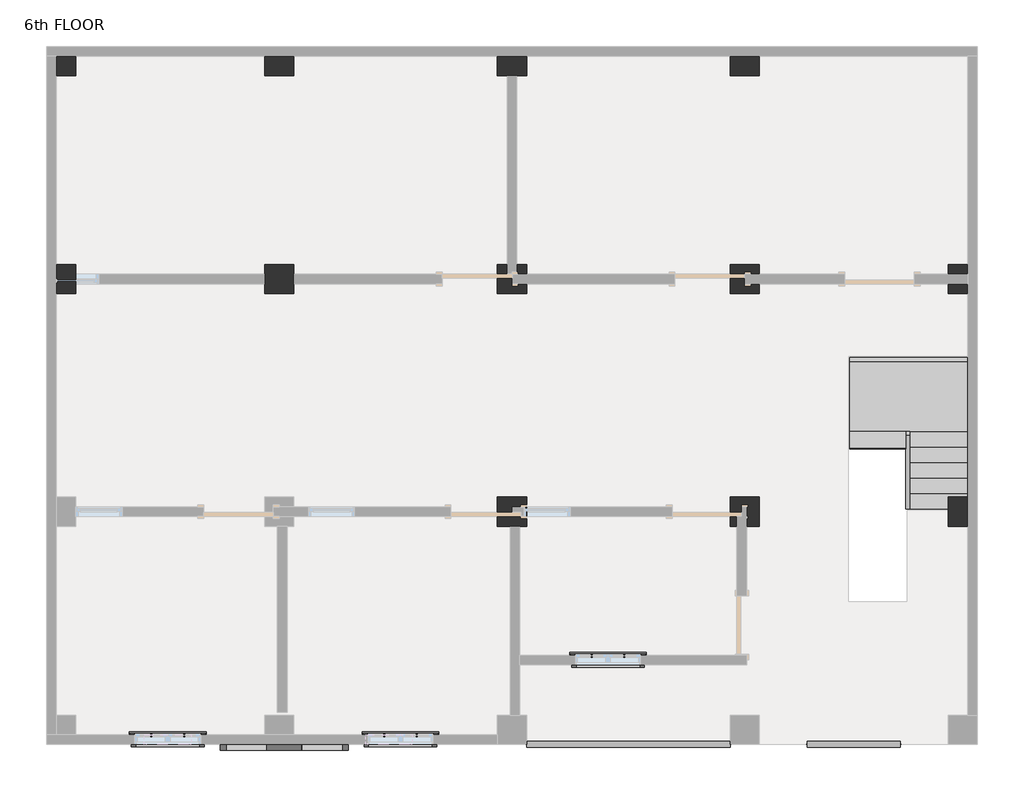
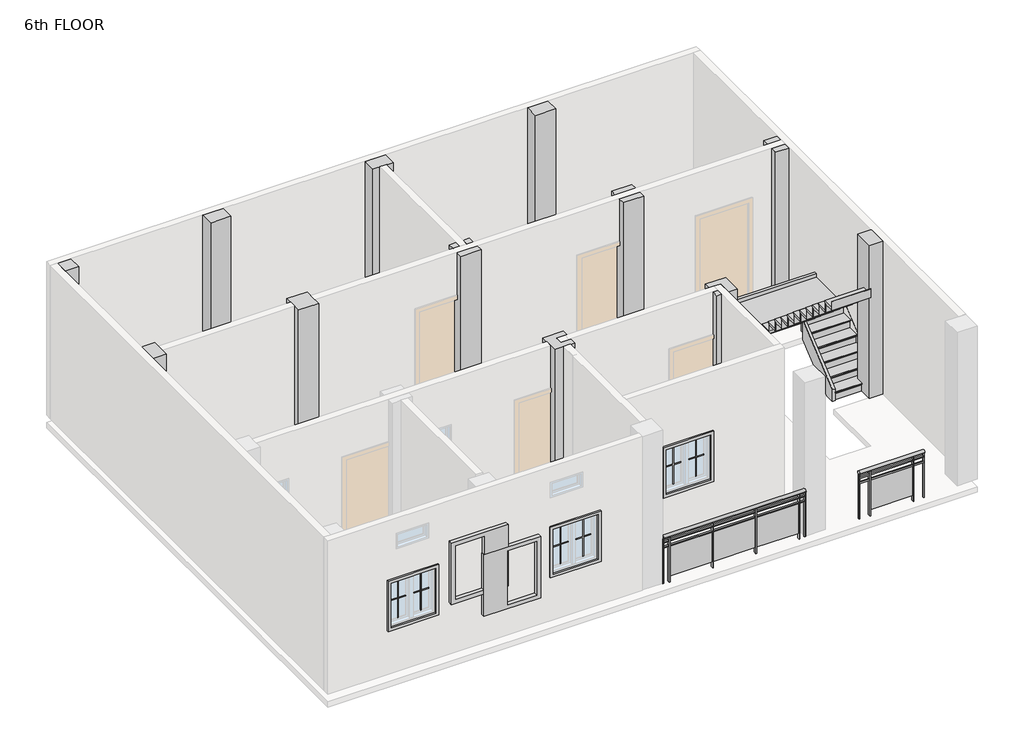
# One storey, part 2 of 2: 12 columns, 12 proxies, 4 members, 2 railings, 1 damper, 1 stair flight.
"""IFC4 building model written with IfcOpenShell, lengths in millimetres."""

from ifc_helpers import new_model, si_unit, point, frame, origin, place, context, project, spatial, polyline, ellipse_curve, trimmed, outline, extrude, faceted_brep, transform, mapped, element, save
from ifc_brep_helpers import plane_surface, extruded_surface, advanced_brep
from components import muntin_pattern_2x2_muntin_pattern_2x2_b3fe6957, muntin_pattern_2x2_muntin_pattern_2x2_3e0ecaf2, trim_window_exterior_flat_with_sill_41619996, trim_window_interior_flat_picture_frame_51c85655, duct_accessories_7_duct_accessories_1_48b7a37f, stair_flight_ae003db1

model = new_model("IFC4")

# Units and contexts
model_context = context("Model", 3, world=origin())
ifc_project = project(units=[si_unit("LENGTHUNIT", "METRE", prefix="MILLI")], contexts=[model_context])

# Site, building, storey
site = spatial("IfcSite", under=ifc_project)
building = spatial("IfcBuilding", under=site)
storey = spatial("IfcBuildingStorey", under=building, Name="6th FLOOR", Elevation=18135.6)

# Proxies
placement = place(None, origin())
muntin_pattern_2x2_muntin_pattern_2x2_shape = muntin_pattern_2x2_muntin_pattern_2x2_b3fe6957(model_context)
element("IfcBuildingElementProxy", 1, Name="Muntin Pattern_2x2 : Muntin Pattern_2x2", ObjectType="Muntin Pattern_2x2 : Muntin Pattern_2x2", at=placement, inside=storey, context=model_context, shape_type="MappedRepresentation", body=[
    mapped(muntin_pattern_2x2_muntin_pattern_2x2_shape, transform((-14441.409625, -253.8184478, 19119.85), x_axis=(1.0, 0.0, 0.0), y_axis=(0.0, 1.0, 0.0), z_axis=(0.0, 0.0, 1.0))),
])
element("IfcBuildingElementProxy", 2, Name="Muntin Pattern_2x2 : Muntin Pattern_2x2", ObjectType="Muntin Pattern_2x2 : Muntin Pattern_2x2", at=placement, inside=storey, context=model_context, shape_type="MappedRepresentation", body=[
    mapped(muntin_pattern_2x2_muntin_pattern_2x2_shape, transform((-11393.409625, -253.8184478, 19119.85), x_axis=(1.0, 0.0, 0.0), y_axis=(0.0, 1.0, 0.0), z_axis=(0.0, 0.0, 1.0))),
])
element("IfcBuildingElementProxy", 3, Name="Muntin Pattern_2x2 : Muntin Pattern_2x2", ObjectType="Muntin Pattern_2x2 : Muntin Pattern_2x2", at=placement, inside=storey, context=model_context, shape_type="MappedRepresentation", body=[
    mapped(muntin_pattern_2x2_muntin_pattern_2x2_shape, transform((-8675.609625, 787.5815522, 19119.85), x_axis=(1.0, 0.0, 0.0), y_axis=(0.0, 1.0, 0.0), z_axis=(0.0, 0.0, 1.0))),
])
muntin_pattern_2x2_muntin_pattern_2x2_2_shape = muntin_pattern_2x2_muntin_pattern_2x2_3e0ecaf2(model_context)
element("IfcBuildingElementProxy", 4, Name="Muntin Pattern_2x2 : Muntin Pattern_2x2", ObjectType="Muntin Pattern_2x2 : Muntin Pattern_2x2", at=placement, inside=storey, context=model_context, shape_type="MappedRepresentation", body=[
    mapped(muntin_pattern_2x2_muntin_pattern_2x2_2_shape, transform((-14012.784625, -253.8184478, 19119.85), x_axis=(-1.0, 0.0, 0.0), y_axis=(0.0, -1.0, 0.0), z_axis=(0.0, 0.0, 1.0))),
])
element("IfcBuildingElementProxy", 5, Name="Muntin Pattern_2x2 : Muntin Pattern_2x2", ObjectType="Muntin Pattern_2x2 : Muntin Pattern_2x2", at=placement, inside=storey, context=model_context, shape_type="MappedRepresentation", body=[
    mapped(muntin_pattern_2x2_muntin_pattern_2x2_2_shape, transform((-10964.784625, -253.8184478, 19119.85), x_axis=(-1.0, 0.0, 0.0), y_axis=(0.0, -1.0, 0.0), z_axis=(0.0, 0.0, 1.0))),
])
element("IfcBuildingElementProxy", 6, Name="Muntin Pattern_2x2 : Muntin Pattern_2x2", ObjectType="Muntin Pattern_2x2 : Muntin Pattern_2x2", at=placement, inside=storey, context=model_context, shape_type="MappedRepresentation", body=[
    mapped(muntin_pattern_2x2_muntin_pattern_2x2_2_shape, transform((-8246.984625, 787.5815522, 19119.85), x_axis=(-1.0, 0.0, 0.0), y_axis=(0.0, -1.0, 0.0), z_axis=(0.0, 0.0, 1.0))),
])
trim_window_exterior_flat_with_sill_shape = trim_window_exterior_flat_with_sill_41619996(model_context)
element("IfcBuildingElementProxy", 7, Name="Trim-Window-Exterior-Flat : with Sill", ObjectType="Trim-Window-Exterior-Flat : with Sill", at=placement, inside=storey, context=model_context, shape_type="MappedRepresentation", body=[
    mapped(trim_window_exterior_flat_with_sill_shape, transform((-14227.097125, -244.2934478, 19964.4), x_axis=(-1.0, 0.0, 0.0), y_axis=(0.0, 0.0, 1.0), z_axis=(0.0, 1.0, 0.0))),
])
element("IfcBuildingElementProxy", 8, Name="Trim-Window-Exterior-Flat : with Sill", ObjectType="Trim-Window-Exterior-Flat : with Sill", at=placement, inside=storey, context=model_context, shape_type="MappedRepresentation", body=[
    mapped(trim_window_exterior_flat_with_sill_shape, transform((-11179.097125, -244.2934478, 19964.4), x_axis=(-1.0, 0.0, 0.0), y_axis=(0.0, 0.0, 1.0), z_axis=(0.0, 1.0, 0.0))),
])
element("IfcBuildingElementProxy", 9, Name="Trim-Window-Exterior-Flat : with Sill", ObjectType="Trim-Window-Exterior-Flat : with Sill", at=placement, inside=storey, context=model_context, shape_type="MappedRepresentation", body=[
    mapped(trim_window_exterior_flat_with_sill_shape, transform((-8461.297125, 797.1065522, 19964.4), x_axis=(-1.0, 0.0, 0.0), y_axis=(0.0, 0.0, 1.0), z_axis=(0.0, 1.0, 0.0))),
])
trim_window_interior_flat_picture_frame_shape = trim_window_interior_flat_picture_frame_51c85655(model_context)
element("IfcBuildingElementProxy", 10, Name="Trim-Window-Interior-Flat : Picture Frame", ObjectType="Trim-Window-Interior-Flat : Picture Frame", at=placement, inside=storey, context=model_context, shape_type="MappedRepresentation", body=[
    mapped(trim_window_interior_flat_picture_frame_shape, transform((-14227.097125, -371.2934478, 19964.4), x_axis=(1.0, 0.0, 0.0), y_axis=(0.0, 0.0, 1.0), z_axis=(0.0, -1.0, 0.0))),
])
element("IfcBuildingElementProxy", 11, Name="Trim-Window-Interior-Flat : Picture Frame", ObjectType="Trim-Window-Interior-Flat : Picture Frame", at=placement, inside=storey, context=model_context, shape_type="MappedRepresentation", body=[
    mapped(trim_window_interior_flat_picture_frame_shape, transform((-11179.097125, -371.2934478, 19964.4), x_axis=(1.0, 0.0, 0.0), y_axis=(0.0, 0.0, 1.0), z_axis=(0.0, -1.0, 0.0))),
])
element("IfcBuildingElementProxy", 12, Name="Trim-Window-Interior-Flat : Picture Frame", ObjectType="Trim-Window-Interior-Flat : Picture Frame", at=placement, inside=storey, context=model_context, shape_type="MappedRepresentation", body=[
    mapped(trim_window_interior_flat_picture_frame_shape, transform((-8461.297125, 670.1065522, 19964.4), x_axis=(1.0, 0.0, 0.0), y_axis=(0.0, 0.0, 1.0), z_axis=(0.0, -1.0, 0.0))),
])

# Columns
element("IfcColumn", 13, ObjectType="column family : column family", at=placement, inside=storey, context=model_context, shape_type="SweptSolid", body=[
    extrude(outline(polyline([(-15433.597125, 8645.7065522), (-15433.597125, 8391.7065522), (-15687.597125, 8391.7065522), (-15687.597125, 8645.7065522), (-15433.597125, 8645.7065522)])), frame((0.0, 0.0, 18140.6), z_axis=(0.0, 0.0, 1.0), x_axis=(1.0, 0.0, 0.0)), (0.0, 0.0, 1.0), 3038.0),
])
element("IfcColumn", 14, ObjectType="column family : column family", at=placement, inside=storey, context=model_context, shape_type="SweptSolid", body=[
    extrude(outline(polyline([(-12576.097125, 5915.2065522), (-12576.097125, 5534.2065522), (-12957.097125, 5534.2065522), (-12957.097125, 5915.2065522), (-12576.097125, 5915.2065522)])), frame((0.0, 0.0, 18140.6), z_axis=(0.0, 0.0, 1.0), x_axis=(1.0, 0.0, 0.0)), (0.0, 0.0, 1.0), 3038.0),
])
element("IfcColumn", 15, ObjectType="column family : column family", at=placement, inside=storey, context=model_context, shape_type="Brep", body=[
    faceted_brep([(-9655.097125, 5915.2065522, 18140.6), (-9528.097125, 5915.2065522, 18140.6), (-9528.097125, 5788.2065522, 18140.6), (-9655.097125, 5788.2065522, 18140.6), (-9528.097125, 5915.2065522, 21178.6), (-9655.097125, 5915.2065522, 21178.6), (-9655.097125, 5788.2065522, 21178.6), (-9528.097125, 5788.2065522, 21178.6)], [[[0, 1, 2, 3]], [[4, 5, 6, 7]], [[0, 3, 6, 5]], [[4, 1, 0, 5]], [[3, 2, 7, 6]], [[1, 4, 7, 2]]]),
    faceted_brep([(-9528.097125, 5534.2065522, 21178.6), (-9528.097125, 5534.2065522, 18140.6), (-9528.097125, 5661.2065522, 18140.6), (-9528.097125, 5661.2065522, 21178.6), (-9909.097125, 5534.2065522, 18140.6), (-9909.097125, 5534.2065522, 21178.6), (-9909.097125, 5915.2065522, 18140.6), (-9909.097125, 5661.2065522, 21178.6), (-9909.097125, 5661.2065522, 20269.2), (-9909.097125, 5788.2065522, 20269.2), (-9909.097125, 5788.2065522, 21178.6), (-9909.097125, 5915.2065522, 21178.6), (-9782.097125, 5915.2065522, 21178.6), (-9782.097125, 5915.2065522, 18140.6), (-9782.097125, 5788.2065522, 18140.6), (-9782.097125, 5788.2065522, 21178.6), (-9782.097125, 5788.2065522, 20269.2), (-9718.597125, 5788.2065522, 18140.6), (-9718.597125, 5788.2065522, 20269.2), (-9718.597125, 5661.2065522, 18140.6), (-9718.597125, 5661.2065522, 20269.2)], [[[0, 1, 2, 3]], [[4, 1, 0, 5]], [[6, 4, 5, 7, 8, 9, 10, 11]], [[6, 11, 12, 13]], [[14, 13, 12, 15, 16]], [[17, 14, 16, 18]], [[19, 20, 8, 7, 3, 2]], [[1, 4, 6, 13, 14, 17, 19, 2]], [[5, 0, 3, 7]], [[12, 11, 10, 15]], [[9, 16, 15, 10]], [[18, 20, 19, 17]], [[20, 18, 16, 9, 8]]]),
])
element("IfcColumn", 16, ObjectType="column family : column family", at=placement, inside=storey, context=model_context, shape_type="Brep", body=[
    faceted_brep([(-6480.097125, 5534.2065522, 18140.6), (-6861.097125, 5534.2065522, 18140.6), (-6861.097125, 5915.2065522, 18140.6), (-6480.097125, 5915.2065522, 18140.6), (-6480.097125, 5788.2065522, 18140.6), (-6670.597125, 5788.2065522, 18140.6), (-6670.597125, 5661.2065522, 18140.6), (-6480.097125, 5661.2065522, 18140.6), (-6480.097125, 5534.2065522, 21178.6), (-6480.097125, 5661.2065522, 21178.6), (-6861.097125, 5534.2065522, 21178.6), (-6861.097125, 5661.2065522, 21178.6), (-6861.097125, 5661.2065522, 20269.2), (-6861.097125, 5788.2065522, 20269.2), (-6861.097125, 5788.2065522, 21178.6), (-6861.097125, 5915.2065522, 21178.6), (-6480.097125, 5915.2065522, 21178.6), (-6670.597125, 5661.2065522, 20269.2), (-6670.597125, 5788.2065522, 20269.2), (-6480.097125, 5788.2065522, 21178.6)], [[[0, 1, 2, 3, 4, 5, 6, 7]], [[8, 0, 7, 9]], [[1, 0, 8, 10]], [[2, 1, 10, 11, 12, 13, 14, 15]], [[3, 2, 15, 16]], [[10, 8, 9, 11]], [[6, 17, 12, 11, 9, 7]], [[13, 18, 5, 4, 19, 14]], [[3, 16, 19, 4]], [[16, 15, 14, 19]], [[18, 17, 6, 5]], [[17, 18, 13, 12]]]),
])
element("IfcColumn", 17, ObjectType="column family : column family", at=placement, inside=storey, context=model_context, shape_type="Brep", body=[
    faceted_brep([(-6480.097125, 2867.2065522, 18140.6), (-6480.097125, 2486.2065522, 18140.6), (-6645.197125, 2486.2065522, 18140.6), (-6645.197125, 2740.2065522, 18140.6), (-6708.697125, 2740.2065522, 18140.6), (-6708.697125, 2613.2065522, 18140.6), (-6772.197125, 2613.2065522, 18140.6), (-6772.197125, 2486.2065522, 18140.6), (-6861.097125, 2486.2065522, 18140.6), (-6861.097125, 2867.2065522, 18140.6), (-6480.097125, 2867.2065522, 21178.6), (-6480.097125, 2486.2065522, 21178.6), (-6861.097125, 2486.2065522, 21178.6), (-6772.197125, 2486.2065522, 21178.6), (-6861.097125, 2613.2065522, 21178.6), (-6861.097125, 2613.2065522, 20269.2), (-6861.097125, 2740.2065522, 20269.2), (-6861.097125, 2740.2065522, 21178.6), (-6861.097125, 2867.2065522, 21178.6), (-6772.197125, 2740.2065522, 21178.6), (-6645.197125, 2740.2065522, 21178.6), (-6645.197125, 2486.2065522, 21178.6), (-6772.197125, 2613.2065522, 21178.6), (-6772.197125, 2613.2065522, 20269.2), (-6772.197125, 2740.2065522, 20269.2), (-6708.697125, 2613.2065522, 20269.2), (-6708.697125, 2740.2065522, 20269.2)], [[[0, 1, 2, 3, 4, 5, 6, 7, 8, 9]], [[1, 0, 10, 11]], [[12, 8, 7, 13]], [[9, 8, 12, 14, 15, 16, 17, 18]], [[0, 9, 18, 10]], [[11, 10, 18, 17, 19, 20, 21]], [[15, 14, 22, 23]], [[17, 16, 24, 19]], [[20, 3, 2, 21]], [[6, 23, 22, 13, 7]], [[14, 12, 13, 22]], [[1, 11, 21, 2]], [[15, 23, 24, 16]], [[25, 23, 6, 5]], [[23, 25, 26, 24]], [[26, 25, 5, 4]], [[24, 26, 4, 3, 20, 19]]]),
])
element("IfcColumn", 18, ObjectType="column family : column family", at=placement, inside=storey, context=model_context, shape_type="Brep", body=[
    faceted_brep([(-9528.097125, 2486.2065522, 18140.6), (-9909.097125, 2486.2065522, 18140.6), (-9909.097125, 2867.2065522, 18140.6), (-9528.097125, 2867.2065522, 18140.6), (-9528.097125, 2740.2065522, 18140.6), (-9566.197125, 2740.2065522, 18140.6), (-9718.597125, 2740.2065522, 18140.6), (-9718.597125, 2613.2065522, 18140.6), (-9566.197125, 2613.2065522, 18140.6), (-9528.097125, 2613.2065522, 18140.6), (-9528.097125, 2486.2065522, 21178.6), (-9528.097125, 2613.2065522, 18440.4), (-9528.097125, 2740.2065522, 18440.4), (-9528.097125, 2867.2065522, 21178.6), (-9528.097125, 2740.2065522, 21178.6), (-9528.097125, 2740.2065522, 20269.2), (-9528.097125, 2613.2065522, 20269.2), (-9528.097125, 2613.2065522, 21178.6), (-9909.097125, 2486.2065522, 21178.6), (-9909.097125, 2867.2065522, 21178.6), (-9566.197125, 2613.2065522, 21178.6), (-9718.597125, 2613.2065522, 21178.6), (-9718.597125, 2740.2065522, 21178.6), (-9566.197125, 2740.2065522, 21178.6), (-9566.197125, 2613.2065522, 20269.2), (-9566.197125, 2613.2065522, 18440.4), (-9566.197125, 2740.2065522, 18440.4), (-9566.197125, 2740.2065522, 20269.2)], [[[0, 1, 2, 3, 4, 5, 6, 7, 8, 9]], [[10, 0, 9, 11, 12, 4, 3, 13, 14, 15, 16, 17]], [[1, 0, 10, 18]], [[2, 1, 18, 19]], [[3, 2, 19, 13]], [[18, 10, 17, 20, 21, 22, 23, 14, 13, 19]], [[11, 9, 8, 7, 21, 20, 17, 16, 24, 25]], [[4, 12, 26, 27, 15, 14, 23, 22, 6, 5]], [[21, 7, 6, 22]], [[25, 24, 27, 26]], [[25, 26, 12, 11]], [[27, 24, 16, 15]]]),
])
element("IfcColumn", 19, ObjectType="column family : column family", at=placement, inside=storey, context=model_context, shape_type="SweptSolid", body=[
    extrude(outline(polyline([(-12576.097125, 8391.7065522), (-12957.097125, 8391.7065522), (-12957.097125, 8645.7065522), (-12576.097125, 8645.7065522), (-12576.097125, 8391.7065522)])), frame((0.0, 0.0, 18140.6), z_axis=(0.0, 0.0, 1.0), x_axis=(1.0, 0.0, 0.0)), (0.0, 0.0, 1.0), 3038.0),
])
element("IfcColumn", 20, ObjectType="column family : column family", at=placement, inside=storey, context=model_context, shape_type="SweptSolid", body=[
    extrude(outline(polyline([(-9528.097125, 8391.7065522), (-9909.097125, 8391.7065522), (-9909.097125, 8645.7065522), (-9528.097125, 8645.7065522), (-9528.097125, 8391.7065522)])), frame((0.0, 0.0, 18140.6), z_axis=(0.0, 0.0, 1.0), x_axis=(1.0, 0.0, 0.0)), (0.0, 0.0, 1.0), 3038.0),
])
element("IfcColumn", 21, ObjectType="column family : column family", at=placement, inside=storey, context=model_context, shape_type="SweptSolid", body=[
    extrude(outline(polyline([(-6480.097125, 8391.7065522), (-6861.097125, 8391.7065522), (-6861.097125, 8645.7065522), (-6480.097125, 8645.7065522), (-6480.097125, 8391.7065522)])), frame((0.0, 0.0, 18140.6), z_axis=(0.0, 0.0, 1.0), x_axis=(1.0, 0.0, 0.0)), (0.0, 0.0, 1.0), 3038.0),
])
element("IfcColumn", 22, ObjectType="column family : column family", at=placement, inside=storey, context=model_context, shape_type="SweptSolid", body=[
    extrude(outline(polyline([(-4003.597125, 5915.2065522), (-3749.597125, 5915.2065522), (-3749.597125, 5788.2065522), (-4003.597125, 5788.2065522), (-4003.597125, 5915.2065522)])), frame((0.0, 0.0, 18140.6), z_axis=(0.0, 0.0, 1.0), x_axis=(1.0, 0.0, 0.0)), (0.0, 0.0, 1.0), 3038.0),
    extrude(outline(polyline([(-3749.597125, 5534.2065522), (-4003.597125, 5534.2065522), (-4003.597125, 5661.2065522), (-3749.597125, 5661.2065522), (-3749.597125, 5534.2065522)])), frame((0.0, 0.0, 18140.6), z_axis=(0.0, 0.0, 1.0), x_axis=(1.0, 0.0, 0.0)), (0.0, 0.0, 1.0), 3038.0),
])
element("IfcColumn", 23, ObjectType="column family : column family", at=placement, inside=storey, context=model_context, shape_type="SweptSolid", body=[
    extrude(outline(polyline([(-4003.597125, 2486.2065522), (-4003.597125, 2867.2065522), (-3749.597125, 2867.2065522), (-3749.597125, 2486.2065522), (-4003.597125, 2486.2065522)])), frame((0.0, 0.0, 18140.6), z_axis=(0.0, 0.0, 1.0), x_axis=(1.0, 0.0, 0.0)), (0.0, 0.0, 1.0), 3038.0),
])
element("IfcColumn", 24, ObjectType="column family : column family", at=placement, inside=storey, context=model_context, shape_type="SweptSolid", body=[
    extrude(outline(polyline([(-15433.597125, 5915.2065522), (-15433.597125, 5534.2065522), (-15687.597125, 5534.2065522), (-15687.597125, 5915.2065522), (-15433.597125, 5915.2065522)])), frame((0.0, 0.0, 18140.6), z_axis=(0.0, 0.0, 1.0), x_axis=(1.0, 0.0, 0.0)), (0.0, 0.0, 1.0), 3038.0),
])

# Damper
duct_accessories_7_duct_accessories_1_shape = duct_accessories_7_duct_accessories_1_48b7a37f(model_context)
element("IfcDamper", 25, ObjectType="Duct Accessories 7 : Duct Accessories 1", at=placement, inside=storey, context=model_context, shape_type="MappedRepresentation", body=[
    mapped(duct_accessories_7_duct_accessories_1_shape, transform((0.0, 0.0, 0.0), x_axis=(1.0, 0.0, 0.0), y_axis=(0.0, 1.0, 0.0), z_axis=(0.0, 0.0, 1.0))),
])

# Members
element("IfcMember", 26, ObjectType="Stringer - 2\" Width", at=placement, inside=storey, context=model_context, shape_type="SweptSolid", body=[
    extrude(outline(polyline([(2714.6319226, 18135.6), (2714.6319226, 18372.4438745), (3679.8319226, 19176.7772078), (3679.8319226, 18780.0165243), (2906.5320935, 18135.6), (2714.6319226, 18135.6)])), frame((-4563.0136682, 0.0, 0.0), z_axis=(1.0, 0.0, 0.0), x_axis=(0.0, 1.0, 0.0)), (0.0, 0.0, 1.0), 50.8),
])
element("IfcMember", 27, ObjectType="Stringer - 2\" Width", at=placement, inside=storey, context=model_context, shape_type="SweptSolid", body=[
    extrude(outline(polyline([(-4512.2136682, 3730.6319226), (-4512.2136682, 3679.8319226), (-4563.0136682, 3679.8319226), (-4563.0136682, 3730.6319226), (-4512.2136682, 3730.6319226)])), frame((0.0, 0.0, 18923.0), z_axis=(0.0, 0.0, 1.0), x_axis=(1.0, 0.0, 0.0)), (0.0, 0.0, 1.0), 304.8),
])
element("IfcMember", 28, ObjectType="Stringer - 2\" Width", at=placement, inside=storey, context=model_context, shape_type="SweptSolid", body=[
    extrude(outline(polyline([(2714.6319226, 18135.6), (2714.6319226, 18372.4438745), (3741.0592732, 19227.8), (4217.1720935, 19227.8), (2906.5320935, 18135.6), (2714.6319226, 18135.6)])), frame((-3749.597125, 0.0, 0.0), z_axis=(1.0, 0.0, 0.0), x_axis=(0.0, 1.0, 0.0)), (0.0, 0.0, 1.0), 50.8),
])
element("IfcMember", 29, ObjectType="Stringer - 2\" Width", at=placement, inside=storey, context=model_context, shape_type="SweptSolid", body=[
    extrude(outline(polyline([(-3698.797125, 4695.8319226), (-3698.797125, 4645.0319226), (-5295.0246464, 4645.0319226), (-5295.0246464, 4695.8319226), (-3698.797125, 4695.8319226)])), frame((0.0, 0.0, 18923.0), z_axis=(0.0, 0.0, 1.0), x_axis=(1.0, 0.0, 0.0)), (0.0, 0.0, 1.0), 304.8),
])

# Railings
element("IfcRailing", 30, ObjectType="Glass Panel - Bottom Fill", at=placement, inside=storey, context=model_context, shape_type="SolidModel", body=[
    advanced_brep(
    [(-9528.097125, -333.1934478, 19050.0), (-9528.097125, -409.3934478, 19050.0), (-6861.097125, -333.1934478, 19050.0), (-6861.097125, -409.3934478, 19050.0)],
    [
        (0, 1, ellipse_curve(frame((-9528.097125, -371.2934478, 19050.0), z_axis=(-1.0, 0.0, 0.0), x_axis=(0.0, -1.0, 0.0)), 38.1, 28.575)),
        (1, 0, ellipse_curve(frame((-9528.097125, -371.2934478, 19050.0), z_axis=(-1.0, 0.0, 0.0), x_axis=(0.0, -1.0, 0.0)), 38.1, 28.575)),
        (2, 3, ellipse_curve(frame((-6861.097125, -371.2934478, 19050.0), z_axis=(1.0, 0.0, 0.0), x_axis=(0.0, -1.0, 0.0)), 38.1, 28.575)),
        (3, 2, ellipse_curve(frame((-6861.097125, -371.2934478, 19050.0), z_axis=(1.0, 0.0, 0.0), x_axis=(0.0, -1.0, 0.0)), 38.1, 28.575)),
        (0, 2),
        (3, 1),
    ],
    [
        plane_surface(frame((-9528.097125, -371.2934478, 19050.0), z_axis=(-1.0, 0.0, 0.0), x_axis=(0.0, 1.0, 0.0))),
        plane_surface(frame((-6861.097125, -371.2934478, 19050.0), z_axis=(1.0, 0.0, 0.0), x_axis=(0.0, 1.0, 0.0))),
        extruded_surface(trimmed(ellipse_curve(frame((-6861.097125, -371.2934478, 19050.0), z_axis=(-1.0, 0.0, 0.0), x_axis=(0.0, -1.0, 0.0)), 38.1, 28.575), [point((-6861.097125, -333.1934478, 19050.0))], [point((-6861.097125, -409.3934478, 19050.0))], True, "CARTESIAN"), (-2667.0, 0.0, 0.0), 2667.0),
        extruded_surface(trimmed(ellipse_curve(frame((-6861.097125, -371.2934478, 19050.0), z_axis=(-1.0, 0.0, 0.0), x_axis=(0.0, -1.0, 0.0)), 38.1, 28.575), [point((-6861.097125, -409.3934478, 19050.0))], [point((-6861.097125, -333.1934478, 19050.0))], True, "CARTESIAN"), (-2667.0, 0.0, 0.0), 2667.0),
    ],
    [
        (0, [[1, 2]]),
        (1, [[3, 4]]),
        (2, [[-1, 5, -4, 6]]),
        (3, [[-2, -6, -3, -5]]),
    ],
),
    extrude(outline(polyline([(-9528.097125, -383.9934478), (-9528.097125, -358.5934478), (-6861.097125, -358.5934478), (-6861.097125, -383.9934478), (-9528.097125, -383.9934478)])), frame((0.0, 0.0, 18935.7), z_axis=(0.0, 0.0, 1.0), x_axis=(1.0, 0.0, 0.0)), (0.0, 0.0, 1.0), 25.4),
    extrude(outline(polyline([(-9528.097125, -383.9934478), (-9528.097125, -358.5934478), (-6861.097125, -358.5934478), (-6861.097125, -383.9934478), (-9528.097125, -383.9934478)])), frame((0.0, 0.0, 18834.1), z_axis=(0.0, 0.0, 1.0), x_axis=(1.0, 0.0, 0.0)), (0.0, 0.0, 1.0), 25.4),
    extrude(outline(polyline([(-6981.747125, -396.6934478), (-6981.747125, -345.8934478), (-6969.047125, -345.8934478), (-6969.047125, -396.6934478), (-6981.747125, -396.6934478)])), frame((0.0, 0.0, 18135.6), z_axis=(0.0, 0.0, 1.0), x_axis=(1.0, 0.0, 0.0)), (0.0, 0.0, 1.0), 885.6788223),
    extrude(outline(polyline([(-7788.197125, -364.7582908), (-6975.397125, -364.7582908), (-6975.397125, -371.1082908), (-7788.197125, -371.1082908), (-7788.197125, -364.7582908)])), frame((0.0, 0.0, 18237.2), z_axis=(0.0, 0.0, 1.0), x_axis=(1.0, 0.0, 0.0)), (0.0, 0.0, 1.0), 596.9),
    extrude(outline(polyline([(-7794.547125, -396.6934478), (-7794.547125, -345.8934478), (-7781.847125, -345.8934478), (-7781.847125, -396.6934478), (-7794.547125, -396.6934478)])), frame((0.0, 0.0, 18135.6), z_axis=(0.0, 0.0, 1.0), x_axis=(1.0, 0.0, 0.0)), (0.0, 0.0, 1.0), 885.6788223),
    extrude(outline(polyline([(-8600.997125, -364.7582908), (-7788.197125, -364.7582908), (-7788.197125, -371.1082908), (-8600.997125, -371.1082908), (-8600.997125, -364.7582908)])), frame((0.0, 0.0, 18237.2), z_axis=(0.0, 0.0, 1.0), x_axis=(1.0, 0.0, 0.0)), (0.0, 0.0, 1.0), 596.9),
    extrude(outline(polyline([(-8607.347125, -396.6934478), (-8607.347125, -345.8934478), (-8594.647125, -345.8934478), (-8594.647125, -396.6934478), (-8607.347125, -396.6934478)])), frame((0.0, 0.0, 18135.6), z_axis=(0.0, 0.0, 1.0), x_axis=(1.0, 0.0, 0.0)), (0.0, 0.0, 1.0), 885.6788223),
    extrude(outline(polyline([(-9413.797125, -364.7582908), (-8600.997125, -364.7582908), (-8600.997125, -371.1082908), (-9413.797125, -371.1082908), (-9413.797125, -364.7582908)])), frame((0.0, 0.0, 18237.2), z_axis=(0.0, 0.0, 1.0), x_axis=(1.0, 0.0, 0.0)), (0.0, 0.0, 1.0), 596.9),
    extrude(outline(polyline([(-9420.147125, -396.6934478), (-9420.147125, -345.8934478), (-9407.447125, -345.8934478), (-9407.447125, -396.6934478), (-9420.147125, -396.6934478)])), frame((0.0, 0.0, 18135.6), z_axis=(0.0, 0.0, 1.0), x_axis=(1.0, 0.0, 0.0)), (0.0, 0.0, 1.0), 885.6788223),
    extrude(outline(polyline([(-6873.797125, -380.8184478), (-6873.797125, -361.7684478), (-6854.747125, -361.7684478), (-6854.747125, -380.8184478), (-6873.797125, -380.8184478)])), frame((0.0, 0.0, 18135.6), z_axis=(0.0, 0.0, 1.0), x_axis=(1.0, 0.0, 0.0)), (0.0, 0.0, 1.0), 885.6788223),
    extrude(outline(polyline([(-9534.447125, -380.8184478), (-9534.447125, -361.7684478), (-9515.397125, -361.7684478), (-9515.397125, -380.8184478), (-9534.447125, -380.8184478)])), frame((0.0, 0.0, 18135.6), z_axis=(0.0, 0.0, 1.0), x_axis=(1.0, 0.0, 0.0)), (0.0, 0.0, 1.0), 885.6788223),
])
element("IfcRailing", 31, ObjectType="Glass Panel - Bottom Fill", at=placement, inside=storey, context=model_context, shape_type="SolidModel", body=[
    advanced_brep(
    [(-5851.447125, -333.1934478, 19050.0), (-5851.447125, -409.3934478, 19050.0), (-4632.247125, -333.1934478, 19050.0), (-4632.247125, -409.3934478, 19050.0)],
    [
        (0, 1, ellipse_curve(frame((-5851.447125, -371.2934478, 19050.0), z_axis=(-1.0, 0.0, 0.0), x_axis=(0.0, -1.0, 0.0)), 38.1, 28.575)),
        (1, 0, ellipse_curve(frame((-5851.447125, -371.2934478, 19050.0), z_axis=(-1.0, 0.0, 0.0), x_axis=(0.0, -1.0, 0.0)), 38.1, 28.575)),
        (2, 3, ellipse_curve(frame((-4632.247125, -371.2934478, 19050.0), z_axis=(1.0, 0.0, 0.0), x_axis=(0.0, -1.0, 0.0)), 38.1, 28.575)),
        (3, 2, ellipse_curve(frame((-4632.247125, -371.2934478, 19050.0), z_axis=(1.0, 0.0, 0.0), x_axis=(0.0, -1.0, 0.0)), 38.1, 28.575)),
        (0, 2),
        (3, 1),
    ],
    [
        plane_surface(frame((-5851.447125, -371.2934478, 19050.0), z_axis=(-1.0, 0.0, 0.0), x_axis=(0.0, 1.0, 0.0))),
        plane_surface(frame((-4632.247125, -371.2934478, 19050.0), z_axis=(1.0, 0.0, 0.0), x_axis=(0.0, 1.0, 0.0))),
        extruded_surface(trimmed(ellipse_curve(frame((-4632.247125, -371.2934478, 19050.0), z_axis=(-1.0, 0.0, 0.0), x_axis=(0.0, -1.0, 0.0)), 38.1, 28.575), [point((-4632.247125, -333.1934478, 19050.0))], [point((-4632.247125, -409.3934478, 19050.0))], True, "CARTESIAN"), (-1219.1999999999998, 0.0, 0.0), 1219.1999999999998),
        extruded_surface(trimmed(ellipse_curve(frame((-4632.247125, -371.2934478, 19050.0), z_axis=(-1.0, 0.0, 0.0), x_axis=(0.0, -1.0, 0.0)), 38.1, 28.575), [point((-4632.247125, -409.3934478, 19050.0))], [point((-4632.247125, -333.1934478, 19050.0))], True, "CARTESIAN"), (-1219.1999999999998, 0.0, 0.0), 1219.1999999999998),
    ],
    [
        (0, [[1, 2]]),
        (1, [[3, 4]]),
        (2, [[-1, 5, -4, 6]]),
        (3, [[-2, -6, -3, -5]]),
    ],
),
    extrude(outline(polyline([(-5851.447125, -383.9934478), (-5851.447125, -358.5934478), (-4632.247125, -358.5934478), (-4632.247125, -383.9934478), (-5851.447125, -383.9934478)])), frame((0.0, 0.0, 18935.7), z_axis=(0.0, 0.0, 1.0), x_axis=(1.0, 0.0, 0.0)), (0.0, 0.0, 1.0), 25.4),
    extrude(outline(polyline([(-5851.447125, -383.9934478), (-5851.447125, -358.5934478), (-4632.247125, -358.5934478), (-4632.247125, -383.9934478), (-5851.447125, -383.9934478)])), frame((0.0, 0.0, 18834.1), z_axis=(0.0, 0.0, 1.0), x_axis=(1.0, 0.0, 0.0)), (0.0, 0.0, 1.0), 25.4),
    extrude(outline(polyline([(-4841.797125, -396.6934478), (-4841.797125, -345.8934478), (-4829.097125, -345.8934478), (-4829.097125, -396.6934478), (-4841.797125, -396.6934478)])), frame((0.0, 0.0, 18135.6), z_axis=(0.0, 0.0, 1.0), x_axis=(1.0, 0.0, 0.0)), (0.0, 0.0, 1.0), 885.6788223),
    extrude(outline(polyline([(-5648.247125, -364.7582908), (-4835.447125, -364.7582908), (-4835.447125, -371.1082908), (-5648.247125, -371.1082908), (-5648.247125, -364.7582908)])), frame((0.0, 0.0, 18237.2), z_axis=(0.0, 0.0, 1.0), x_axis=(1.0, 0.0, 0.0)), (0.0, 0.0, 1.0), 596.9),
    extrude(outline(polyline([(-5654.597125, -396.6934478), (-5654.597125, -345.8934478), (-5641.897125, -345.8934478), (-5641.897125, -396.6934478), (-5654.597125, -396.6934478)])), frame((0.0, 0.0, 18135.6), z_axis=(0.0, 0.0, 1.0), x_axis=(1.0, 0.0, 0.0)), (0.0, 0.0, 1.0), 885.6788223),
    extrude(outline(polyline([(-4644.947125, -380.8184478), (-4644.947125, -361.7684478), (-4625.897125, -361.7684478), (-4625.897125, -380.8184478), (-4644.947125, -380.8184478)])), frame((0.0, 0.0, 18135.6), z_axis=(0.0, 0.0, 1.0), x_axis=(1.0, 0.0, 0.0)), (0.0, 0.0, 1.0), 885.6788223),
    extrude(outline(polyline([(-5857.797125, -380.8184478), (-5857.797125, -361.7684478), (-5838.747125, -361.7684478), (-5838.747125, -380.8184478), (-5857.797125, -380.8184478)])), frame((0.0, 0.0, 18135.6), z_axis=(0.0, 0.0, 1.0), x_axis=(1.0, 0.0, 0.0)), (0.0, 0.0, 1.0), 885.6788223),
])

# Stair flight
stair_flight_shape = stair_flight_ae003db1(model_context)
element("IfcStairFlight", 32, ObjectType="2\" Tread 1\" Nosing 1/4\" Riser", at=placement, inside=storey, context=model_context, shape_type="MappedRepresentation", body=[
    mapped(stair_flight_shape, transform((0.0, 0.0, 0.0), x_axis=(1.0, 0.0, 0.0), y_axis=(0.0, 1.0, 0.0), z_axis=(0.0, 0.0, 1.0))),
])

save(model, "model.ifc")

# Revit data of these elements
# Type "Muntin Pattern_2x2 : Muntin Pattern_2x2"
#   Width [instance default] = 4' - 0"
#   Thickness = 0' - 0 1/2"
#   Height [instance default] = 4' - 0"
#   Distance = 0' - 0 3/4"
#   Interior Material [instance default] = none
#   Exterior Material [instance default] = none
#   Default Elevation = 0
# Type "Trim-Window-Exterior-Flat : with Sill"
#   Trim Width = 0' - 2 1/4"
#   Trim Thickness_Picture Frame = 0' - 1 1/4"
#   Trim Thickness_with Sill = 0' - 0 3/4"
#   Sill Thickness = 0' - 1 1/4"
#   Opening Width [instance default] = 2' - 0"
#   Opening Height [instance default] = 3' - 0"
#   Default Elevation = 4' - 0"
#   Sill = yes
#   Picture Frame = no
#   Trim Material [instance default] = none
# Type "Trim-Window-Interior-Flat : Picture Frame"
#   Trim Thickness_Picture Frame = 0' - 1 1/4"
#   Trim Width = 0' - 2 1/4"
#   Trim Thickness_with Sill = 0' - 0 3/4"
#   Sill Thickness = 0' - 1 1/4"
#   Opening Width [instance default] = 2' - 0"
#   Opening Height [instance default] = 3' - 0"
#   Default Elevation = 4' - 0"
#   Sill = no
#   Picture Frame = yes
#   Trim Material [instance default] = none
# Type "column family : column family"
#   w2 [instance default] = 0' - 9.88189"
#   w1 [instance default] = 0' - 9.01575"
#   Depth = 1' - 11.62205"
#   Width = 1' - 11.62205"
# Type "Glass Panel - Bottom Fill"
#   Assembly Code = "C2010400"
#   built-in parameter 1008612 = 0.0416667 (stored number, unit not read)
#   built-in parameter 1008611 = 0.0416667 (stored number, unit not read)
#   built-in parameter 1008609 = 0.333333 (stored number, unit not read)
#   built-in parameter 1008604 = 0.166667 (stored number, unit not read)
#   built-in parameter 1008603 = 0.166667 (stored number, unit not read)
#   Railing Height = 3' - 0"
#   built-in parameter 1008630 = 2
#   built-in parameter 1008610 = 2
#   built-in parameter 1008618 = Baluster - Square : 3/4"
# Elements 1, 2, 3, 4, 5, 6 (IfcBuildingElementProxy, "Muntin Pattern_2x2 : Muntin Pattern_2x2")
#   Width = 0' - 11 5/8"
#   Height = 2' - 6 1/2"
#   Interior Material = Wood - Stained
#   Exterior Material = Clad - White
#   Phase Created = New Construction
#   Materials on its faces: "Clad - White", "Wood - Stained"
# Elements 7, 8, 9 (IfcBuildingElementProxy, "Trim-Window-Exterior-Flat : with Sill")
#   Opening Width = 2' - 10"
#   Opening Height = 3' - 0"
#   Trim Material = Clad - White
#   Phase Created = New Construction
#   Materials on its faces: "Clad - White"
# Elements 10, 11, 12 (IfcBuildingElementProxy, "Trim-Window-Interior-Flat : Picture Frame")
#   Opening Width = 2' - 10"
#   Opening Height = 3' - 0"
#   Trim Material = Wood - Stained
#   Phase Created = New Construction
#   Materials on its faces: "Wood - Stained"
# Elements 13, 14, 15, 19, 20, 21 (IfcColumn, "column family : column family")
#   w2 = 1' - 3"
#   w1 = 1' - 3"
#   Phase Created = New Construction
#   Materials on its faces: "Default Wall"
# Elements 16, 22, 23 (IfcColumn, "column family : column family")
#   w2 = 1' - 3"
#   w1 = 1' - 3"
#   Phase Created = New Construction
#   Materials on its faces: "grey", "Default Wall"
# Elements 17, 18 (IfcColumn, "column family : column family")
#   w2 = 1' - 3"
#   w1 = 1' - 3"
#   Phase Created = New Construction
#   Materials on its faces: "Default Wall", "inside wall"
# Element 24 (IfcColumn, "column family : column family")
#   w2 = 1' - 3"
#   w1 = 1' - 3"
#   Phase Created = New Construction
#   Materials on its faces: "inside wall", "Default Wall"
# Element 25 (IfcDamper, "Duct Accessories 7 : Duct Accessories 1")
#   Mark = "7"
#   Phase Created = New Construction
#   Materials on its faces: "border"
# Elements 26, 27, 28, 29 (IfcMember, "Stringer - 2\" Width")
#   Phase Created = New Construction
# Elements 30, 31 (IfcRailing, "Glass Panel - Bottom Fill")
#   Phase Created = New Construction
#   Materials on its faces: "Glass"
# Element 32 (IfcStairFlight, "2\" Tread 1\" Nosing 1/4\" Riser")
#   Phase Created = New Construction
# Materials
#   "Clad - White": class "Wood", colour RGB 242 242 238, transparency 0, Cost = 0
#   "Wood - Stained": class "Wood", colour RGB 224 178 126, transparency 0, Cost = 0
#   "Default Wall": colour RGB 128 128 128, transparency 0, Cost = 0
#   "grey": class "Generic", colour RGB 80 80 80, transparency 0, Cost = 0
#   "inside wall": class "Generic", colour RGB 199 224 95, transparency 0, Cost = 0
#   "border": class "Generic", colour RGB 144 144 144, transparency 0, Cost = 0
#   "Glass": class "Glass", colour RGB 0 128 192, transparency 0.75, Description = "Soda Lime Glass", Cost = 0
